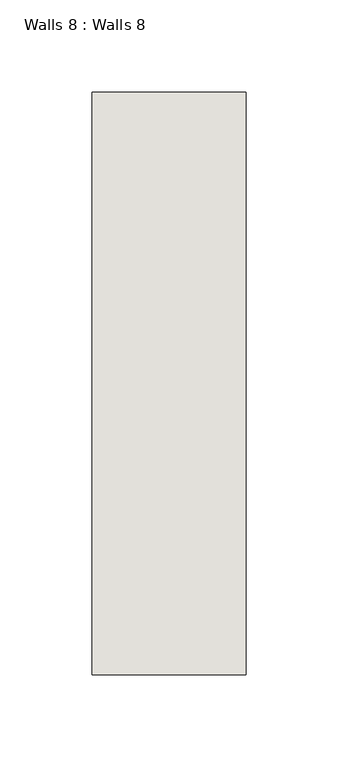
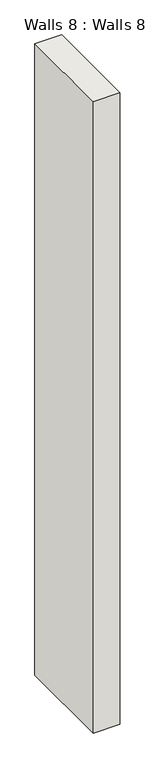
"""IFC4 building model written with IfcOpenShell, lengths in millimetres: wall geometry, Walls 8 : Walls 8."""

from ifc_helpers import new_model, si_unit, frame, origin, place, context, project, spatial, polyline, outline, extrude, source, transform, mapped, element, save


def walls_8_walls_8_394d44dd(model_context):
    return source(origin(), model_context, "Body", "SweptSolid", [
        extrude(outline(polyline([(-3344.2530528, -17647.4508748), (-3427.5361288, -17647.4508748), (-3427.5361288, -17331.9685282), (-3344.2530528, -17331.9685282), (-3344.2530528, -17647.4508748)])), frame((0.0, 0.0, -54.1554296), z_axis=(0.0, 0.0, 1.0), x_axis=(1.0, 0.0, 0.0)), (0.0, 0.0, 1.0), 2082.8),
    ])


if __name__ == "__main__":
    model = new_model("IFC4")
    model_context = context("Model", 3, world=origin())
    ifc_project = project(units=[si_unit("LENGTHUNIT", "METRE", prefix="MILLI")], contexts=[model_context])
    site = spatial("IfcSite", under=ifc_project)
    building = spatial("IfcBuilding", under=site)
    placement = place(None, origin())
    walls_8_walls_8_shape = walls_8_walls_8_394d44dd(model_context)
    element("IfcWall", 1, ObjectType="Walls 8 : Walls 8", at=placement, inside=building, context=model_context, shape_type="MappedRepresentation", body=[
        mapped(walls_8_walls_8_shape, transform((0.0, 0.0, 0.0), x_axis=(1.0, 0.0, 0.0), y_axis=(0.0, 1.0, 0.0), z_axis=(0.0, 0.0, 1.0))),
    ])
    save(model, "model.ifc")

# Revit data of these elements
# Element 1 (IfcWall, "Walls 8 : Walls 8")
#   Materials on its faces: "Door - Frame", "Default Wall"
# Materials
#   "Door - Frame": colour RGB 118 70 51, transparency 0
#   "Default Wall": colour RGB 128 128 128, transparency 0
